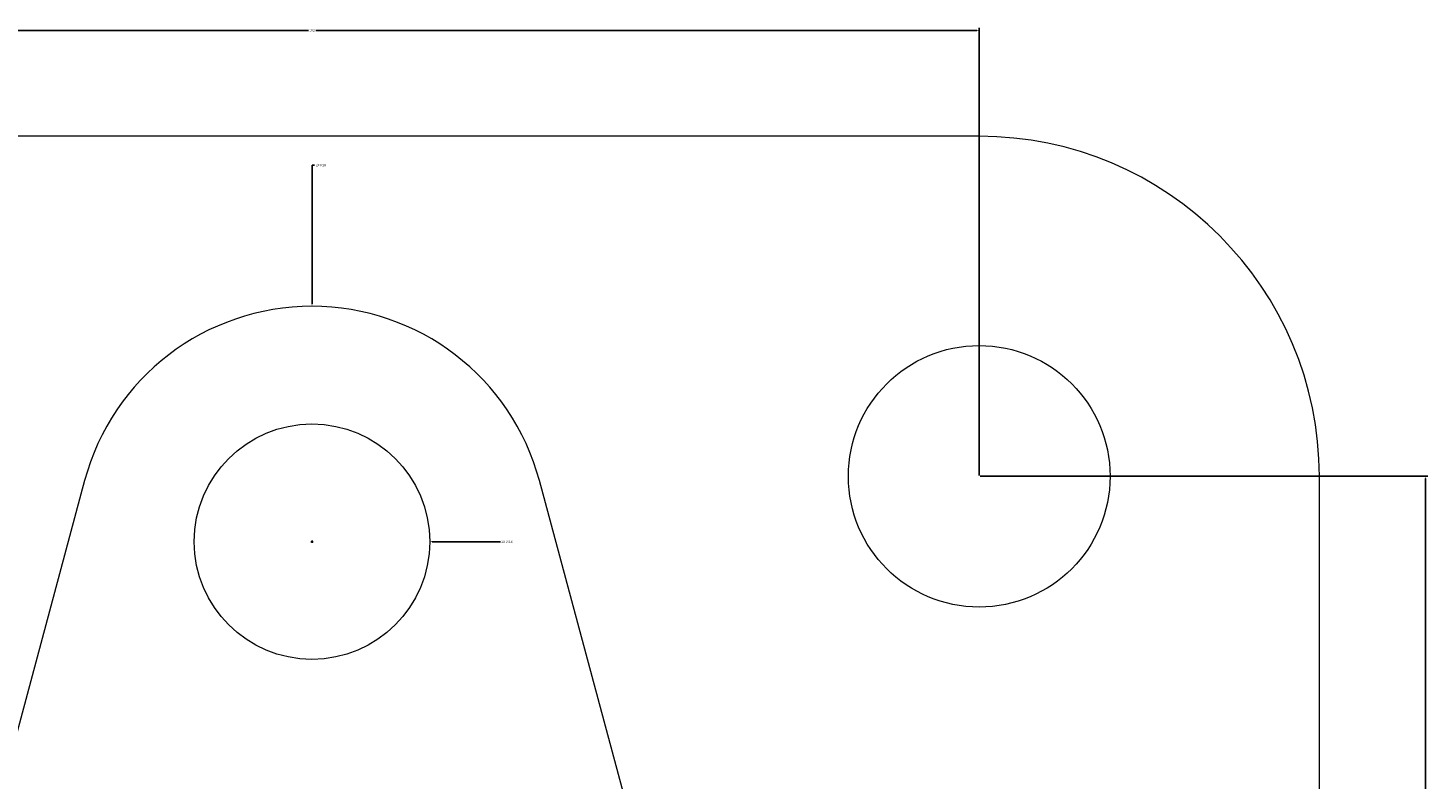
# Model space of a CAD drawing. Units: millimetres. Extents: x 2597 to 2768, y 1809 to 1980.
# Tile 7 of 7: x 2661 to 2768, y 1922 to 1980. Entities that reach past the tile are written whole.
import ezdxf

# ---------------------------------------------------------------- set-up
doc = ezdxf.new("R2010")
doc.units = ezdxf.units.MM
doc.layers.add('M-CONS', color=8, linetype='Continuous', lineweight=18)
doc.layers.add('M-DIMS', color=2, linetype='Continuous', lineweight=18)
doc.styles.get("Standard").update_dxf_attribs({"font": 'arial.ttf'})
doc.dimstyles.get("Standard").update_dxf_attribs({"dimtxt": 0.18, "dimasz": 0.18, "dimexe": 0.18, "dimexo": 0.0625, "dimgap": 0.09, "dimtad": 0, "dimtih": 1, "dimtoh": 1, "dimdec": 4, "dimzin": 0, "dimdsep": 46, "dimtxsty": 'Standard', "dimcen": 0.09, "dimadec": 0, "dimazin": 0, "dimtfac": 1, "dimtdec": 4, "dimtofl": 0, "dimtmove": 0, "dimatfit": 3, "dimfxl": 1, "dimtolj": 1, "dimtzin": 0, "dimarcsym": 0})

# ---------------------------------------------------------------- blocks, each defined once
blk = doc.blocks.new('*D5')
at = {"layer": 'Defpoints', "color": 0, "transparency": 16777216}
for p in [(2733.78, 1979.53), (2631.78, 1945.43), (2733.78, 1945.43)]:
    blk.add_point(p, dxfattribs=at)
at = {"layer": 'M-DIMS', "color": 0, "lineweight": -2, "transparency": 16777216}
for p, q in [((2631.78, 1945.49), (2631.78, 1979.71)), ((2733.78, 1945.49), (2733.78, 1979.71)), ((2631.96, 1979.53), (2682.5, 1979.53)), ((2733.6, 1979.53), (2683.06, 1979.53))]:
    blk.add_line(p, q, dxfattribs=at)
at = {"layer": 'M-DIMS', "color": 0, "transparency": 16777216}
for points in [[(2631.96, 1979.56), (2631.96, 1979.5), (2631.78, 1979.53)], [(2733.6, 1979.56), (2733.6, 1979.5), (2733.78, 1979.53)]]:
    blk.add_solid(points, dxfattribs=at)
at = {"layer": 'M-DIMS', "color": 0, "transparency": 16777216, "insert": (2682.78, 1979.53), "char_height": 0.18, "attachment_point": 5}
blk.add_mtext('\\A1;102', dxfattribs=at)
blk = doc.blocks.new('*D6')
at = {"layer": 'Defpoints', "color": 0, "transparency": 16777216}
for p in [(2733.78, 1945.43), (2767.88, 1945.43), (2733.78, 1843.43)]:
    blk.add_point(p, dxfattribs=at)
at = {"layer": 'M-DIMS', "color": 0, "lineweight": -2, "transparency": 16777216}
for p, q in [((2733.84, 1945.43), (2768.06, 1945.43)), ((2767.88, 1945.25), (2767.88, 1894.61)), ((2767.88, 1843.61), (2767.88, 1894.25)), ((2733.84, 1843.43), (2768.06, 1843.43))]:
    blk.add_line(p, q, dxfattribs=at)
at = {"layer": 'M-DIMS', "color": 0, "transparency": 16777216}
for points in [[(2767.85, 1945.25), (2767.91, 1945.25), (2767.88, 1945.43)], [(2767.85, 1843.61), (2767.91, 1843.61), (2767.88, 1843.43)]]:
    blk.add_solid(points, dxfattribs=at)
at = {"layer": 'M-DIMS', "color": 0, "transparency": 16777216, "insert": (2767.88, 1894.43), "char_height": 0.18, "attachment_point": 5}
blk.add_mtext('\\A1;102', dxfattribs=at)
blk = doc.blocks.new('*D17')
at = {"layer": 'Defpoints', "color": 0, "transparency": 16777216}
for p in [(2682.78, 1958.43), (2682.78, 1940.43)]:
    blk.add_point(p, dxfattribs=at)
at = {"layer": 'M-DIMS', "color": 0, "lineweight": -2, "transparency": 16777216}
for p, q in [((2682.96, 1969.23), (2682.78, 1969.23)), ((2682.78, 1969.23), (2682.78, 1958.61)), ((2682.69, 1940.43), (2682.87, 1940.43)), ((2682.78, 1940.34), (2682.78, 1940.52))]:
    blk.add_line(p, q, dxfattribs=at)
at = {"layer": 'M-DIMS', "color": 0, "transparency": 16777216}
blk.add_solid([(2682.75, 1958.61), (2682.81, 1958.61), (2682.78, 1958.43)], dxfattribs=at)
at = {"layer": 'M-DIMS', "color": 0, "transparency": 16777216, "insert": (2683.46, 1969.23), "char_height": 0.18, "attachment_point": 5}
blk.add_mtext('\\A1;2X R18', dxfattribs=at)
blk = doc.blocks.new('*D18')
at = {"layer": 'Defpoints', "color": 0, "transparency": 16777216}
for p in [(2673.78, 1940.43), (2691.78, 1940.43)]:
    blk.add_point(p, dxfattribs=at)
at = {"layer": 'M-DIMS', "color": 0, "lineweight": -2, "transparency": 16777216}
for p, q in [((2682.69, 1940.43), (2682.87, 1940.43)), ((2682.78, 1940.34), (2682.78, 1940.52)), ((2697.18, 1940.43), (2691.96, 1940.43))]:
    blk.add_line(p, q, dxfattribs=at)
at = {"layer": 'M-DIMS', "color": 0, "transparency": 16777216}
blk.add_solid([(2691.96, 1940.46), (2691.96, 1940.4), (2691.78, 1940.43)], dxfattribs=at)
at = {"layer": 'M-DIMS', "color": 0, "transparency": 16777216, "insert": (2697.68, 1940.43), "char_height": 0.18, "attachment_point": 5}
blk.add_mtext('\\A1;2X ∅18', dxfattribs=at)

msp = doc.modelspace()

# ---------------------------------------------------------------- linework, layer by layer
at = {"layer": 'M-CONS'}
msp.add_lwpolyline([(2631.7756, 1817.4301), (2733.7756, 1817.4301, 0.41421356), (2759.7756, 1843.4301), (2759.7756, 1945.4301, 0.41421356), (2733.7756, 1971.4301), (2631.7756, 1971.4301, 0.41421356), (2605.7756, 1945.4301), (2605.7756, 1843.4301, 0.41421356)], format="xyb", close=True, dxfattribs=at)
msp.add_lwpolyline([(2713.7756, 1903.4301), (2745.7756, 1903.4301), (2745.7756, 1913.4301), (2708.6698, 1913.4301), (2700.1588, 1945.1014, 0.76675137), (2665.3923, 1945.1014), (2656.8814, 1913.4301), (2619.7756, 1913.4301), (2619.7756, 1903.4301), (2651.7756, 1903.4301), (2651.7756, 1885.4301), (2619.7756, 1885.4301), (2619.7756, 1875.4301), (2656.8814, 1875.4301), (2665.3923, 1843.7587, 0.76675137), (2700.1588, 1843.7587), (2708.6698, 1875.4301), (2745.7756, 1875.4301), (2745.7756, 1885.4301), (2713.7756, 1885.4301), (2713.7756, 1903.4301), (2713.7756, 1894.4301)], format="xyb", dxfattribs=at)
for centre, radius in [((2733.7756, 1945.4301), 10), ((2682.7756, 1940.4301), 9)]:
    msp.add_circle(centre, radius, dxfattribs=at)

# ---------------------------------------------------------------- dimensions: what is measured, and where the dimension line sits
at = {"layer": 'M-DIMS'}
dim = msp.add_linear_dim(base=(2733.7756, 1979.5301), p1=(2631.7756, 1945.4301), p2=(2733.7756, 1945.4301), dimstyle='Standard', override={"dimdec": 0, "dimlfac": 1, "dimrnd": 0, "dimzin": 0, "dimdsep": 46, "dimlunit": 2}, dxfattribs=at)
dim.commit()
dim.dimension.update_dxf_attribs({"geometry": '*D5', "text_midpoint": (2682.7756, 1979.5301)})
dim = msp.add_radius_dim(center=(2682.7756, 1940.4301), mpoint=(2682.776, 1958.4301), text='2X <>', dimstyle='Standard', override={"dimdec": 0, "dimlfac": 1, "dimrnd": 0, "dimzin": 0, "dimdsep": 46, "dimlunit": 2}, dxfattribs=at)
dim.commit()
dim.dimension.update_dxf_attribs({"geometry": '*D17', "text_midpoint": (2683.4564, 1969.2301), "dimtype": 164})
dim = msp.add_linear_dim(base=(2767.8756, 1945.4301), p1=(2733.7756, 1843.4301), p2=(2733.7756, 1945.4301), angle=90, dimstyle='Standard', override={"dimdec": 0, "dimlfac": 1, "dimrnd": 0, "dimzin": 0, "dimdsep": 46, "dimlunit": 2}, dxfattribs=at)
dim.commit()
dim.dimension.update_dxf_attribs({"geometry": '*D6', "text_midpoint": (2767.8756, 1894.4301)})
dim = msp.add_diameter_dim_2p(p1=(2673.7756, 1940.4302), p2=(2691.7756, 1940.43), text='2X <>', dimstyle='Standard', override={"dimdec": 0, "dimlfac": 1, "dimrnd": 0, "dimzin": 0, "dimdsep": 46, "dimlunit": 2}, dxfattribs=at)
dim.commit()
dim.dimension.update_dxf_attribs({"geometry": '*D18', "text_midpoint": (2697.1756, 1940.4299), "dimtype": 163})

doc.saveas('drawing.dxf')
